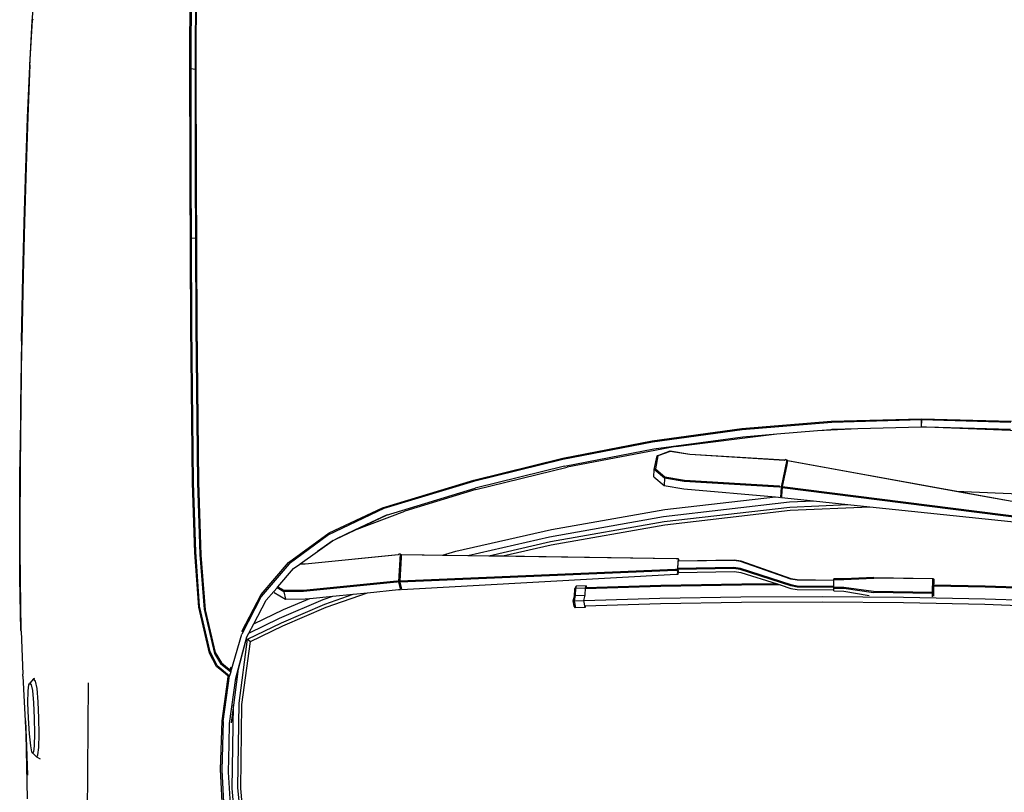
# Model space of a CAD drawing. Units: inches. Extents: x 22042254 to 25404563, y 17568978 to 17626777.
# Tile 32 of 45: x 22179810 to 22179853, y 17626332 to 17626366. Entities that reach past the tile are written whole.
import ezdxf

# ---------------------------------------------------------------- set-up
doc = ezdxf.new("R2010")
doc.units = ezdxf.units.IN
doc.header["$MEASUREMENT"] = 0
doc.layers.add('A-SITE-VEHI', color=8, linetype='Continuous', lineweight=18)
doc.layers.add('Edges', color=250, linetype='Continuous')

# ---------------------------------------------------------------- blocks, each defined once
blk = doc.blocks.new('Nissan Qashqai pl')
at = {"layer": 'Edges'}
for p, q in [((8.43872, 12.06738), (8.43593, 11.9861)), ((8.43969, 12.06744), (8.4369, 11.98609)), ((8.45166, 12.06738), (8.44886, 11.98585)), ((8.45405, 11.98566), (8.45684, 12.06694)), ((8.34061, 11.95665), (8.34476, 12.05358)), ((8.35747, 12.04752), (8.31037, 11.78808)), ((8.37023, 12.0427), (8.33738, 11.78256)), ((8.35648, 11.87066), (8.37461, 12.04353)), ((8.33603, 11.78277), (8.36877, 12.04191)), ((8.27648, 11.92734), (8.28039, 12.03052)), ((8.26824, 11.92208), (8.27079, 12.01226)), ((8.27192, 12.01183), (8.26946, 11.92208)), ((8.27648, 11.92734), (8.27881, 12.01143)), ((8.34061, 11.95665), (8.34946, 12.00531)), ((8.43593, 11.9861), (8.43483, 11.93464)), ((8.4369, 11.98609), (8.4358, 11.93462)), ((8.44886, 11.98585), (8.44712, 11.90427)), ((8.45232, 11.90432), (8.45405, 11.98566)), ((8.31, 11.78823), (8.34061, 11.95665)), ((8.42721, 11.87457), (8.42809, 11.93355)), ((8.42868, 11.93352), (8.4278, 11.87454)), ((8.42809, 11.93355), (8.42904, 11.93453)), ((8.42809, 11.93355), (8.42871, 11.93358)), ((8.42868, 11.93352), (8.42809, 11.93355)), ((8.42871, 11.93358), (8.42868, 11.93352)), ((8.44184, 11.93322), (8.42868, 11.93352)), ((8.42904, 11.93453), (8.42871, 11.93358)), ((8.43281, 11.93469), (8.42904, 11.93453)), ((8.42904, 11.93453), (8.43257, 11.93445)), ((8.43281, 11.93469), (8.43257, 11.93445)), ((8.43257, 11.93445), (8.43483, 11.9344)), ((8.43483, 11.93464), (8.43281, 11.93469)), ((8.43483, 11.93464), (8.43483, 11.9344)), ((8.4358, 11.93462), (8.43483, 11.93464)), ((8.43483, 11.9344), (8.4358, 11.93438)), ((8.4358, 11.93462), (8.4358, 11.93438)), ((8.4459, 11.9344), (8.4358, 11.93462)), ((8.4358, 11.93438), (8.44219, 11.93423)), ((8.44184, 11.93322), (8.44219, 11.93423)), ((8.44219, 11.93423), (8.4459, 11.9344)), ((8.44219, 11.93423), (8.44312, 11.93321)), ((8.4459, 11.9344), (8.44594, 11.93439)), ((8.27632, 11.92228), (8.27644, 11.92631)), ((8.27644, 11.92631), (8.27648, 11.92734)), ((8.44096, 11.87424), (8.44184, 11.93322)), ((8.44312, 11.93321), (8.44184, 11.93322)), ((8.44312, 11.93321), (8.44224, 11.87423)), ((8.44645, 11.93335), (8.44312, 11.93321)), ((8.27079, 11.83191), (8.26824, 11.92208)), ((8.27632, 11.92228), (8.26946, 11.92208)), ((8.26946, 11.92208), (8.27633, 11.92188)), ((8.26946, 11.92208), (8.27192, 11.83233)), ((8.27633, 11.92188), (8.27632, 11.92228)), ((8.27812, 11.8585), (8.27633, 11.92188)), ((8.44712, 11.90427), (8.44644, 11.82272)), ((8.45164, 11.82302), (8.45232, 11.90432)), ((8.42721, 11.87457), (8.42864, 11.84454)), ((8.42924, 11.8445), (8.4278, 11.87454)), ((8.35415, 11.8485), (8.35648, 11.87066)), ((8.35992, 11.79058), (8.35648, 11.87066)), ((8.43675, 11.84433), (8.44096, 11.87424)), ((8.43803, 11.84433), (8.44224, 11.87423)), ((8.44077, 11.84444), (8.44521, 11.86984)), ((8.28002, 11.81804), (8.27812, 11.8585)), ((8.27881, 11.83273), (8.27812, 11.8585)), ((8.27888, 11.8319), (8.27812, 11.8585)), ((8.35053, 11.81394), (8.35415, 11.8485)), ((8.35665, 11.79034), (8.35415, 11.8485)), ((8.42864, 11.84454), (8.42849, 11.83454)), ((8.42909, 11.83451), (8.42924, 11.8445)), ((8.43661, 11.83454), (8.43675, 11.84433)), ((8.43789, 11.83451), (8.43803, 11.84433)), ((8.44062, 11.83445), (8.44077, 11.84444)), ((8.2781, 11.74232), (8.27079, 11.83191)), ((8.27192, 11.83233), (8.27932, 11.74259)), ((8.27888, 11.8319), (8.27881, 11.83273)), ((8.28002, 11.81804), (8.27888, 11.8319)), ((8.42909, 11.83451), (8.42849, 11.83454)), ((8.42977, 11.83449), (8.42909, 11.83451)), ((8.42923, 11.79785), (8.42977, 11.83449)), ((8.43037, 11.83448), (8.42977, 11.83449)), ((8.43037, 11.83448), (8.42983, 11.79781)), ((8.43601, 11.83435), (8.43037, 11.83448)), ((8.43545, 11.79769), (8.43601, 11.83435)), ((8.4366, 11.83434), (8.43601, 11.83435)), ((8.4366, 11.83437), (8.43661, 11.83454)), ((8.43729, 11.83437), (8.4366, 11.83437)), ((8.43729, 11.83437), (8.4366, 11.83434)), ((8.4366, 11.83434), (8.4366, 11.83437)), ((8.43661, 11.83454), (8.43789, 11.83451)), ((8.43729, 11.83437), (8.43674, 11.79768)), ((8.43789, 11.83439), (8.43729, 11.83437)), ((8.43789, 11.83433), (8.43729, 11.83437)), ((8.43789, 11.83439), (8.43789, 11.83451)), ((8.43968, 11.83441), (8.43789, 11.83433)), ((8.43789, 11.83433), (8.43789, 11.83439)), ((8.43914, 11.79778), (8.43968, 11.83441)), ((8.44062, 11.83445), (8.43968, 11.83441)), ((8.2834, 11.7773), (8.28002, 11.81804)), ((8.44644, 11.82272), (8.44682, 11.74128)), ((8.452, 11.74183), (8.45164, 11.82302)), ((8.34718, 11.78206), (8.35053, 11.81394)), ((8.35156, 11.78997), (8.35053, 11.81394)), ((8.4281, 11.79144), (8.42923, 11.79785)), ((8.42983, 11.79781), (8.42873, 11.79139)), ((8.43435, 11.79124), (8.43545, 11.79769)), ((8.43674, 11.79768), (8.43568, 11.79124)), ((8.43812, 11.79141), (8.43914, 11.79778)), ((8.30918, 11.78629), (8.30935, 11.78727)), ((8.30918, 11.78629), (8.30987, 11.78513)), ((8.30951, 11.78528), (8.30918, 11.78629)), ((8.30935, 11.78727), (8.33672, 11.78161)), ((8.31591, 11.78693), (8.30935, 11.78727)), ((8.31, 11.78823), (8.31037, 11.78808)), ((8.31037, 11.78808), (8.31591, 11.78693)), ((8.31591, 11.78693), (8.33603, 11.78277)), ((8.36623, 11.66386), (8.35156, 11.78997)), ((8.37126, 11.66453), (8.35665, 11.79034)), ((8.37452, 11.66499), (8.35992, 11.79058)), ((8.41069, 11.74115), (8.4281, 11.79144)), ((8.42873, 11.79139), (8.41111, 11.74099)), ((8.41791, 11.74061), (8.43435, 11.79124)), ((8.43568, 11.79124), (8.4193, 11.74067)), ((8.43467, 11.78052), (8.43812, 11.79141)), ((8.29596, 11.67617), (8.2834, 11.7773)), ((8.28622, 11.74339), (8.2834, 11.7773)), ((8.3038, 11.69029), (8.30951, 11.78528)), ((8.30987, 11.78513), (8.30416, 11.69014)), ((8.32983, 11.68483), (8.33554, 11.77982)), ((8.33688, 11.77961), (8.33118, 11.68463)), ((8.33554, 11.77982), (8.33656, 11.78063)), ((8.33603, 11.78277), (8.33738, 11.78256)), ((8.33672, 11.78161), (8.33656, 11.78063)), ((8.33656, 11.78063), (8.33688, 11.77961)), ((8.33672, 11.78161), (8.34702, 11.78107)), ((8.33738, 11.78256), (8.34062, 11.7824)), ((8.33853, 11.68425), (8.34643, 11.77614)), ((8.34583, 11.78132), (8.34062, 11.7824)), ((8.34062, 11.7824), (8.34574, 11.78213)), ((8.34583, 11.78132), (8.34574, 11.78213)), ((8.34574, 11.78213), (8.34718, 11.78206)), ((8.34702, 11.78107), (8.34583, 11.78132)), ((8.34643, 11.77614), (8.34668, 11.7791)), ((8.35927, 11.66508), (8.34643, 11.77614)), ((8.34668, 11.7791), (8.34702, 11.78107)), ((8.42225, 11.74131), (8.43371, 11.77751)), ((8.43371, 11.77751), (8.43467, 11.78052)), ((8.43371, 11.77751), (8.43387, 11.74228)), ((8.43467, 11.78052), (8.43484, 11.74209)), ((8.29048, 11.65238), (8.2781, 11.74232)), ((8.27932, 11.74259), (8.29164, 11.65284)), ((8.2985, 11.65403), (8.28622, 11.74339)), ((8.40967, 11.73479), (8.41069, 11.74115)), ((8.41111, 11.74099), (8.41004, 11.73462)), ((8.41696, 11.73421), (8.41791, 11.74061)), ((8.4193, 11.74067), (8.41833, 11.73428)), ((8.42133, 11.73497), (8.42225, 11.74131)), ((8.43387, 11.74228), (8.43527, 11.66128)), ((8.43484, 11.74209), (8.43625, 11.66103)), ((8.44682, 11.74128), (8.44824, 11.66004)), ((8.45342, 11.66083), (8.452, 11.74183)), ((8.41042, 11.67906), (8.40967, 11.73479)), ((8.41004, 11.73462), (8.41078, 11.67914)), ((8.41773, 11.67797), (8.41696, 11.73421)), ((8.41833, 11.73428), (8.41909, 11.67804)), ((8.42208, 11.67874), (8.42133, 11.73497)), ((8.30047, 11.67062), (8.3038, 11.69029)), ((8.30416, 11.69014), (8.30092, 11.67045)), ((8.32641, 11.66517), (8.32983, 11.68483)), ((8.33118, 11.68463), (8.32784, 11.66495)), ((8.3352, 11.66457), (8.33853, 11.68425)), ((8.40819, 11.67854), (8.41042, 11.67906)), ((8.40819, 11.67854), (8.40856, 11.67837)), ((8.40822, 11.67656), (8.40819, 11.67854)), ((8.40856, 11.67837), (8.40859, 11.67639)), ((8.40856, 11.67837), (8.4117, 11.67819)), ((8.41042, 11.67906), (8.41078, 11.67914)), ((8.41043, 11.67855), (8.41042, 11.67906)), ((8.41079, 11.67864), (8.41043, 11.67855)), ((8.41043, 11.67855), (8.41079, 11.67838)), ((8.41078, 11.67914), (8.41079, 11.67864)), ((8.41079, 11.67864), (8.41079, 11.67838)), ((8.41079, 11.67838), (8.4117, 11.67833)), ((8.4117, 11.67833), (8.4117, 11.67819)), ((8.4117, 11.67833), (8.41773, 11.67797)), ((8.4117, 11.67819), (8.41896, 11.67775)), ((8.41773, 11.67797), (8.41909, 11.67804)), ((8.41896, 11.67775), (8.42033, 11.67782)), ((8.41899, 11.67577), (8.41896, 11.67775)), ((8.41909, 11.67804), (8.42208, 11.67874)), ((8.42382, 11.67863), (8.42033, 11.67782)), ((8.42033, 11.67782), (8.42036, 11.67583)), ((8.42382, 11.67863), (8.42208, 11.67874)), ((8.42385, 11.67665), (8.42382, 11.67863)), ((8.29596, 11.67617), (8.31658, 11.56748)), ((8.30531, 11.65739), (8.30047, 11.67062)), ((8.30092, 11.67045), (8.30545, 11.65831)), ((8.40859, 11.67639), (8.40451, 11.40111)), ((8.40565, 11.50276), (8.40822, 11.67656)), ((8.43052, 11.39957), (8.41899, 11.67577)), ((8.42036, 11.67583), (8.43188, 11.39963)), ((8.43936, 11.40138), (8.42385, 11.67665)), ((8.30545, 11.65831), (8.30531, 11.65739)), ((8.319, 11.65456), (8.30531, 11.65739)), ((8.30545, 11.65831), (8.31822, 11.65566)), ((8.31822, 11.65566), (8.32641, 11.66517)), ((8.32784, 11.66495), (8.319, 11.65456)), ((8.32635, 11.65418), (8.3352, 11.66457)), ((8.32784, 11.66495), (8.3352, 11.66457)), ((8.37916, 11.55154), (8.35927, 11.66508)), ((8.38635, 11.54971), (8.36623, 11.66386)), ((8.39129, 11.55062), (8.37126, 11.66453)), ((8.39454, 11.55127), (8.37452, 11.66499)), ((8.43527, 11.66128), (8.43753, 11.5863)), ((8.43625, 11.66103), (8.43851, 11.58581)), ((8.44824, 11.66004), (8.45053, 11.58434)), ((8.45569, 11.58548), (8.45342, 11.66083)), ((8.30764, 11.56315), (8.29048, 11.65238)), ((8.29164, 11.65284), (8.3089, 11.5631)), ((8.31566, 11.56466), (8.2985, 11.65403)), ((8.319, 11.65456), (8.31822, 11.65566)), ((8.32635, 11.65418), (8.319, 11.65456)), ((8.43769, 11.58568), (8.43573, 11.58638)), ((8.43573, 11.58638), (8.43592, 11.57648)), ((8.43573, 11.58638), (8.43753, 11.5863)), ((8.43753, 11.5863), (8.43753, 11.58616)), ((8.43788, 11.57578), (8.43769, 11.58568)), ((8.44503, 11.58535), (8.43769, 11.58568)), ((8.44522, 11.57545), (8.44503, 11.58535)), ((8.45034, 11.58408), (8.44503, 11.58535)), ((8.45725, 11.58541), (8.45034, 11.58408)), ((8.45053, 11.57418), (8.45034, 11.58408)), ((8.45569, 11.58548), (8.45725, 11.58541)), ((8.45569, 11.58534), (8.45569, 11.58548)), ((8.45725, 11.58541), (8.45744, 11.57551)), ((8.43592, 11.57648), (8.43788, 11.57578)), ((8.43592, 11.57648), (8.43771, 11.57526)), ((8.43869, 11.57491), (8.43771, 11.57526)), ((8.43788, 11.57578), (8.44522, 11.57545)), ((8.4384, 11.57523), (8.44569, 11.5749)), ((8.44596, 11.57458), (8.43869, 11.57491)), ((8.44522, 11.57545), (8.45053, 11.57418)), ((8.45072, 11.57344), (8.44596, 11.57458)), ((8.45053, 11.57418), (8.45744, 11.57551)), ((8.45072, 11.57344), (8.45053, 11.57418)), ((8.45588, 11.57444), (8.45072, 11.57344)), ((8.45744, 11.57551), (8.45588, 11.57444)), ((8.32965, 11.4739), (8.30764, 11.56315)), ((8.3089, 11.5631), (8.33108, 11.47335)), ((8.31566, 11.56466), (8.33775, 11.47528)), ((8.33915, 11.47576), (8.31658, 11.56748)), ((8.40094, 11.45586), (8.37916, 11.55154)), ((8.40513, 11.46781), (8.38635, 11.54971)), ((8.40544, 11.48873), (8.39129, 11.55062)), ((8.40565, 11.50276), (8.39454, 11.55127)), ((8.40544, 11.48873), (8.40565, 11.50276)), ((8.40513, 11.46781), (8.40544, 11.48873)), ((8.35734, 11.38238), (8.32965, 11.4739)), ((8.33108, 11.47335), (8.3582, 11.3836)), ((8.36476, 11.38628), (8.33775, 11.47528)), ((8.33915, 11.47576), (8.36083, 11.40481)), ((8.40475, 11.44233), (8.40513, 11.46781)), ((8.40475, 11.44233), (8.40094, 11.45586)), ((8.40415, 11.40128), (8.40475, 11.44233)), ((8.3799, 11.35447), (8.36083, 11.40481)), ((8.40704, 11.40096), (8.40366, 11.40017)), ((8.40415, 11.40128), (8.40451, 11.40111)), ((8.40451, 11.40111), (8.40704, 11.40096)), ((8.40704, 11.40096), (8.43052, 11.39957)), ((8.43598, 11.40059), (8.43936, 11.40138)), ((8.40366, 11.40017), (8.4314, 11.39852)), ((8.40367, 11.39919), (8.40366, 11.40017)), ((8.40367, 11.39919), (8.40455, 11.39814)), ((8.40419, 11.39831), (8.40367, 11.39919)), ((8.41345, 11.30495), (8.40419, 11.39831)), ((8.40455, 11.39814), (8.41382, 11.30478)), ((8.43052, 11.39957), (8.43188, 11.39963)), ((8.43056, 11.39659), (8.43141, 11.39753)), ((8.43982, 11.30323), (8.43056, 11.39659)), ((8.4314, 11.39852), (8.43937, 11.40038)), ((8.4314, 11.39852), (8.43141, 11.39753)), ((8.43141, 11.39753), (8.43193, 11.39666)), ((8.43188, 11.39963), (8.43598, 11.40059)), ((8.43193, 11.39666), (8.44119, 11.3033)), ((8.43937, 11.40038), (8.43598, 11.40059)), ((8.4394, 11.3984), (8.43937, 11.40038)), ((8.44249, 11.36723), (8.4394, 11.3984)), ((8.3826, 11.32909), (8.35734, 11.38238)), ((8.3582, 11.3836), (8.38444, 11.32843)), ((8.36461, 11.38699), (8.3799, 11.35447)), ((8.38882, 11.33551), (8.36476, 11.38628)), ((8.45708, 11.3258), (8.44249, 11.36723)), ((8.44389, 11.35313), (8.44249, 11.36723)), ((8.3799, 11.35447), (8.38882, 11.33551)), ((8.45396, 11.32453), (8.44389, 11.35313)), ((8.44593, 11.33263), (8.44389, 11.35313)), ((8.39008, 11.33285), (8.38882, 11.33551)), ((8.39008, 11.33285), (8.40108, 11.3173)), ((8.39041, 11.33215), (8.39008, 11.33285)), ((8.40108, 11.3173), (8.39041, 11.33215)), ((8.44935, 11.32292), (8.44593, 11.33263)), ((8.44822, 11.30945), (8.44593, 11.33263)), ((8.41218, 11.28832), (8.3826, 11.32909)), ((8.38444, 11.32843), (8.41339, 11.28877)), ((8.46803, 11.27933), (8.44935, 11.32292)), ((8.47252, 11.28116), (8.45396, 11.32453)), ((8.47556, 11.28265), (8.45708, 11.3258)), ((8.41352, 11.29999), (8.40108, 11.3173)), ((8.41352, 11.29999), (8.41345, 11.30495)), ((8.41382, 11.30478), (8.41391, 11.29944)), ((8.44, 11.2834), (8.43982, 11.30323)), ((8.44119, 11.3033), (8.44145, 11.28346)), ((8.45936, 11.28311), (8.44822, 11.30945)), ((8.44866, 11.30504), (8.44822, 11.30945)), ((8.44893, 11.28521), (8.44866, 11.30504)), ((8.41391, 11.29944), (8.41352, 11.29999)), ((8.41829, 11.29335), (8.41391, 11.29944)), ((8.43651, 11.27757), (8.41829, 11.29335)), ((8.44441, 11.26076), (8.41218, 11.28832)), ((8.41339, 11.28877), (8.44622, 11.26088)), ((8.43651, 11.27757), (8.44, 11.2834)), ((8.44145, 11.28346), (8.43748, 11.27673)), ((8.44145, 11.28346), (8.44893, 11.28521)), ((8.44216, 11.27372), (8.44893, 11.28521)), ((8.47371, 11.25336), (8.45936, 11.28311)), ((8.49139, 11.24998), (8.47556, 11.28265)), ((8.43748, 11.27673), (8.43651, 11.27757)), ((8.44121, 11.2735), (8.43748, 11.27673)), ((8.44216, 11.27372), (8.44121, 11.2735)), ((8.44994, 11.26593), (8.44121, 11.2735)), ((8.48305, 11.24842), (8.46803, 11.27933)), ((8.48894, 11.2473), (8.47252, 11.28116)), ((8.47371, 11.25336), (8.44994, 11.26593)), ((8.48142, 11.2413), (8.44441, 11.26076)), ((8.44622, 11.26088), (8.48381, 11.24147)), ((8.48305, 11.24842), (8.47371, 11.25336)), ((8.48667, 11.24651), (8.48305, 11.24842)), ((8.52797, 11.23535), (8.48667, 11.24651)), ((8.52142, 11.23743), (8.48667, 11.24651)), ((8.48894, 11.2473), (8.49139, 11.24998)), ((8.55313, 11.23871), (8.48894, 11.2473)), ((8.55442, 11.24156), (8.49139, 11.24998)), ((8.74806, 11.24732), (8.6375, 11.23757)), ((8.74909, 11.25014), (8.63861, 11.24043)), ((8.52164, 11.2303), (8.48381, 11.24147)), ((8.52142, 11.23743), (8.55498, 11.23301)), ((8.53014, 11.23516), (8.52142, 11.23743)), ((8.57356, 11.22909), (8.52797, 11.23535)), ((8.6375, 11.23757), (8.55313, 11.23871)), ((8.63861, 11.24043), (8.55442, 11.24156)), ((8.6721, 11.23482), (8.63869, 11.23189)), ((8.51253, 11.22103), (8.51766, 11.22719)), ((8.5132, 11.2202), (8.52164, 11.2303)), ((8.51552, 11.21677), (8.5258, 11.22907)), ((8.52367, 11.22522), (8.51632, 11.21624)), ((8.51971, 11.22969), (8.51661, 11.23068)), ((8.51766, 11.22719), (8.51971, 11.22969)), ((8.52164, 11.2303), (8.51971, 11.22969)), ((8.52164, 11.2303), (8.5258, 11.22907)), ((8.52592, 11.22792), (8.52367, 11.22522)), ((8.5258, 11.22907), (8.52592, 11.22792)), ((8.57154, 11.22268), (8.5258, 11.22907)), ((8.52937, 11.22743), (8.52592, 11.22792)), ((8.57063, 11.2216), (8.52937, 11.22743)), ((8.63869, 11.23189), (8.55498, 11.23301)), ((8.55498, 11.23301), (8.57261, 11.23069)), ((8.59415, 11.22865), (8.57356, 11.22909)), ((8.59406, 11.22889), (8.59415, 11.22865)), ((8.62205, 11.22805), (8.59415, 11.22865)), ((8.62035, 11.2213), (8.6721, 11.22407)), ((8.66989, 11.23098), (8.62205, 11.22805)), ((8.45884, 11.20363), (8.50324, 11.21407)), ((8.45947, 11.20468), (8.50247, 11.21481)), ((8.51552, 11.21677), (8.50181, 11.20976)), ((8.50247, 11.21481), (8.51253, 11.22103)), ((8.51632, 11.21624), (8.50294, 11.20916)), ((8.50324, 11.21407), (8.5132, 11.2202)), ((8.61967, 11.2201), (8.57063, 11.2216)), ((8.57154, 11.22268), (8.62035, 11.2213)), ((8.66831, 11.22263), (8.61967, 11.2201)), ((8.40486, 11.20045), (8.45947, 11.20468)), ((8.50181, 11.20976), (8.45586, 11.19911)), ((8.50294, 11.20916), (8.45708, 11.1983)), ((7.82329, 11.1958), (7.90142, 11.19549)), ((7.82329, 11.19498), (7.90204, 11.19468)), ((7.90142, 11.19549), (7.91849, 11.19552)), ((7.90204, 11.19468), (7.91833, 11.1947)), ((7.91833, 11.1947), (7.9176, 11.19075)), ((7.91849, 11.19552), (7.91833, 11.1947)), ((7.91833, 11.1947), (8.02749, 11.19482)), ((7.91849, 11.19552), (8.02732, 11.19568)), ((8.02732, 11.19568), (8.17527, 11.1963)), ((8.02749, 11.19482), (8.08756, 11.19507)), ((8.08756, 11.19507), (8.08729, 11.1911)), ((8.08756, 11.19507), (8.17541, 11.19543)), ((8.17527, 11.1963), (8.33175, 11.19799)), ((8.17541, 11.19543), (8.33197, 11.19709)), ((8.33175, 11.19799), (8.40486, 11.20045)), ((8.33197, 11.19709), (8.40425, 11.19948)), ((8.40141, 11.19533), (8.33242, 11.19312)), ((8.40223, 11.19434), (8.33243, 11.19203)), ((8.45586, 11.19911), (8.40141, 11.19533)), ((8.45708, 11.1983), (8.40223, 11.19434)), ((8.40425, 11.19948), (8.45884, 11.20363)), ((7.90396, 11.18944), (7.80829, 11.18979)), ((7.90357, 11.19074), (7.82329, 11.19107)), ((7.9176, 11.19075), (7.90357, 11.19074)), ((8.02759, 11.18962), (7.90396, 11.18944)), ((8.0275, 11.19086), (7.9176, 11.19075)), ((8.08729, 11.1911), (8.0275, 11.19086)), ((8.17534, 11.1903), (8.02759, 11.18962)), ((8.17546, 11.19146), (8.08729, 11.1911)), ((8.33243, 11.19203), (8.17534, 11.1903)), ((8.33242, 11.19312), (8.17546, 11.19146)), ((8.53262, 11.08741), (8.66752, 11.0866)), ((8.53854, 11.0363), (8.53103, 11.03463)), ((8.55176, 11.03752), (8.53854, 11.0363)), ((8.56796, 11.03824), (8.55176, 11.03752)), ((8.58417, 11.03842), (8.56796, 11.03824)), ((8.5974, 11.03808), (8.58417, 11.03842)), ((8.60494, 11.03726), (8.5974, 11.03808)), ((8.60732, 11.03618), (8.60325, 11.03208)), ((8.60732, 11.03618), (8.60494, 11.03726)), ((8.60903, 11.03968), (8.60732, 11.03618)), ((7.86997, 11.03154), (7.83812, 11.0342)), ((7.86805, 11.03202), (7.86903, 11.03174)), ((7.91369, 11.02919), (7.86903, 11.03174)), ((7.91514, 11.02896), (7.86997, 11.03154)), ((7.91369, 11.02919), (7.96577, 11.02701)), ((7.96683, 11.02681), (7.91514, 11.02896)), ((7.96577, 11.02701), (8.01597, 11.02528)), ((8.01677, 11.0251), (7.96683, 11.02681)), ((8.5283, 11.03362), (8.52871, 11.03293)), ((8.53103, 11.03463), (8.52871, 11.03293)), ((8.52871, 11.03293), (8.5331, 11.02921)), ((8.5331, 11.02921), (8.53458, 11.03031)), ((8.53467, 11.02825), (8.5331, 11.02921)), ((8.53458, 11.03031), (8.54056, 11.03164)), ((8.54067, 11.02743), (8.53467, 11.02825)), ((8.54056, 11.03164), (8.55262, 11.03277)), ((8.55273, 11.02727), (8.54067, 11.02743)), ((8.55262, 11.03277), (8.5681, 11.0335)), ((8.56822, 11.02778), (8.55273, 11.02727)), ((8.5681, 11.0335), (8.58359, 11.03372)), ((8.58372, 11.02881), (8.56822, 11.02778)), ((8.58359, 11.03372), (8.59567, 11.03343)), ((8.59581, 11.03009), (8.58372, 11.02881)), ((8.58379, 11.02511), (8.64892, 11.0263)), ((8.59567, 11.03343), (8.6017, 11.03277)), ((8.6018, 11.03125), (8.59581, 11.03009)), ((8.59646, 11.02576), (8.62518, 11.02679)), ((8.6017, 11.03277), (8.60325, 11.03208)), ((8.60325, 11.03208), (8.6018, 11.03125)), ((8.01597, 11.02528), (8.07131, 11.02365)), ((8.07176, 11.02351), (8.01677, 11.0251)), ((8.07131, 11.02365), (8.1249, 11.02232)), ((8.12514, 11.02218), (8.07176, 11.02351)), ((8.1249, 11.02232), (8.19007, 11.02098)), ((8.19016, 11.02085), (8.12514, 11.02218)), ((8.19007, 11.02098), (8.19375, 11.02096)), ((8.19015, 11.02104), (8.19375, 11.02096)), ((8.1904, 11.02085), (8.19016, 11.02085)), ((8.1904, 11.02085), (8.25433, 11.01983)), ((8.19375, 11.02096), (8.19538, 11.02093)), ((8.19538, 11.02093), (8.25438, 11.01996)), ((8.25444, 11.01983), (8.25433, 11.01985)), ((8.25433, 11.01983), (8.25444, 11.01983)), ((8.25438, 11.01996), (8.31663, 11.0193)), ((8.25444, 11.01983), (8.25564, 11.01981)), ((8.25564, 11.01981), (8.25601, 11.01983)), ((8.25601, 11.01983), (8.25612, 11.01983)), ((8.25612, 11.01983), (8.26926, 11.01967)), ((8.26926, 11.01967), (8.26936, 11.01967)), ((8.26936, 11.01967), (8.30977, 11.01919)), ((8.30977, 11.01919), (8.31627, 11.01918)), ((8.36626, 11.019), (8.31627, 11.01918)), ((8.35975, 11.01896), (8.31627, 11.01918)), ((8.31663, 11.0193), (8.37641, 11.01907)), ((8.36023, 11.01896), (8.35975, 11.01896)), ((8.36077, 11.01896), (8.36023, 11.01896)), ((8.36626, 11.019), (8.36077, 11.01896)), ((8.36626, 11.019), (8.37641, 11.01907)), ((8.37572, 11.01896), (8.36626, 11.019)), ((8.4282, 11.01925), (8.37572, 11.01896)), ((8.37641, 11.01907), (8.40688, 11.01923)), ((8.40688, 11.01923), (8.42186, 11.01955)), ((8.40688, 11.01923), (8.42917, 11.01934)), ((8.47991, 11.02025), (8.4282, 11.01925)), ((8.42917, 11.01934), (8.47991, 11.02025)), ((8.48109, 11.02031), (8.47991, 11.02025)), ((8.48109, 11.02031), (8.52408, 11.02198)), ((8.5259, 11.0221), (8.52408, 11.02198)), ((8.5259, 11.0221), (8.58379, 11.02511)), ((8.5707, 11.02484), (8.59646, 11.02576)), ((8.58379, 11.02511), (8.59646, 11.02576))]:
    blk.add_line(p, q, dxfattribs=at)
blk = doc.blocks.new('CAR')
blk.add_blockref('Nissan Qashqai pl', (-9.74328, -11.91512))

msp = doc.modelspace()

# ---------------------------------------------------------------- block references
at = {"layer": 'A-SITE-VEHI', "xscale": 43.56002006885659, "yscale": 43.56002006885659, "zscale": 43.56002006885659, "rotation": 270}
msp.add_blockref('CAR', (22179848.861, 17626284.325), dxfattribs=at)

doc.saveas('drawing.dxf')
